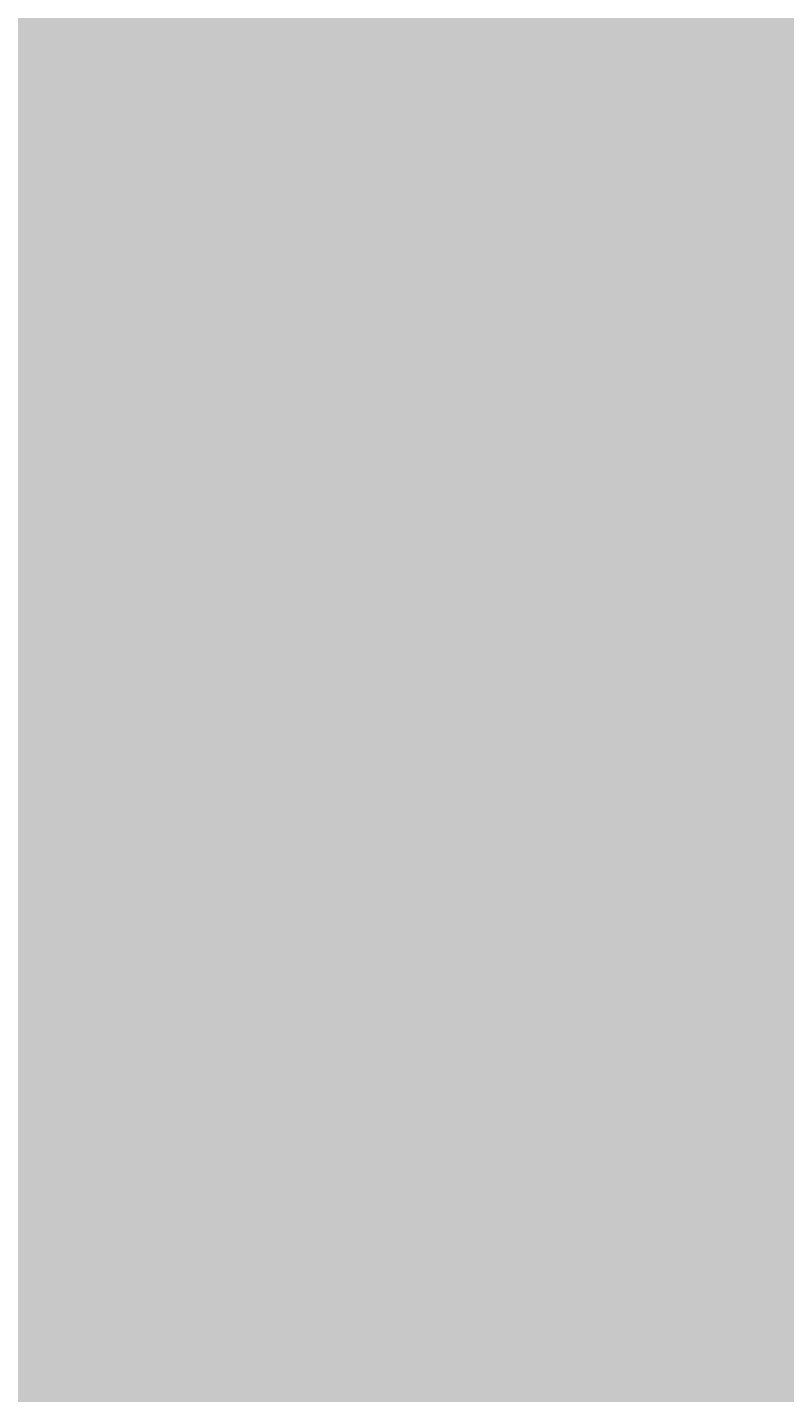
# Model space of a CAD drawing. Units: inches. Extents: x 84 to 1044, y -280 to 906.
# Tile 98 of 105: x 826 to 861, y 445 to 510. Entities that reach past the tile are written whole.
import ezdxf

# ---------------------------------------------------------------- set-up
doc = ezdxf.new("R2010")
doc.units = ezdxf.units.IN
doc.layers.add('A-ANNO-DIMS', color=2, linetype='Continuous', lineweight=18)
doc.layers.add('L-PLNT-PATT', color=9, linetype='Continuous', lineweight=9, true_color=0xafd9aa)
doc.styles.get("Standard").update_dxf_attribs({"font": 'arial.ttf'})
doc.dimstyles.get("Standard").update_dxf_attribs({"dimtxt": 0.18, "dimasz": 0.18, "dimexe": 0.18, "dimexo": 0.0625, "dimgap": 0.09, "dimtad": 0, "dimtih": 1, "dimtoh": 1, "dimdec": 4, "dimzin": 0, "dimdsep": 46, "dimtxsty": 'Standard', "dimcen": 0.09, "dimadec": 0, "dimazin": 0, "dimtfac": 1, "dimtdec": 4, "dimtofl": 0, "dimtmove": 0, "dimatfit": 3, "dimfxl": 1, "dimtolj": 1, "dimtzin": 0, "dimarcsym": 0})

# ---------------------------------------------------------------- blocks, each defined once
blk = doc.blocks.new('*D62')
at = {"layer": 'A-ANNO-DIMS', "color": 0, "lineweight": -2, "transparency": 16777216}
for p, q in [((203.179, 709.183), (203.179, 905.9)), ((203.359, 905.72), (549.232, 905.72)), ((895.894, 905.72), (550.021, 905.72)), ((896.074, 400.183), (896.074, 905.9))]:
    blk.add_line(p, q, dxfattribs=at)
at = {"layer": 'A-ANNO-DIMS', "color": 0, "transparency": 16777216}
for points in [[(203.359, 905.75), (203.359, 905.69), (203.179, 905.72)], [(895.894, 905.75), (895.894, 905.69), (896.074, 905.72)]]:
    blk.add_solid(points, dxfattribs=at)
at = {"layer": 'Defpoints', "color": 0, "transparency": 16777216}
for p in [(896.074, 905.72), (203.179, 709.12), (896.074, 400.12)]:
    blk.add_point(p, dxfattribs=at)
at = {"layer": 'A-ANNO-DIMS', "color": 0, "transparency": 16777216, "insert": (549.627, 905.72), "char_height": 0.18, "attachment_point": 5}
blk.add_mtext('\\A1;692.9', dxfattribs=at)
blk = doc.blocks.new('*D63')
at = {"layer": 'A-ANNO-DIMS', "color": 0, "lineweight": -2, "transparency": 16777216}
for p, q in [((833.136, 709.12), (1043.768, 709.12)), ((1043.588, 708.94), (1043.588, 400.302)), ((1043.588, 91.3), (1043.588, 399.938)), ((896.136, 91.12), (1043.768, 91.12))]:
    blk.add_line(p, q, dxfattribs=at)
at = {"layer": 'A-ANNO-DIMS', "color": 0, "transparency": 16777216}
for points in [[(1043.558, 708.94), (1043.618, 708.94), (1043.588, 709.12)], [(1043.558, 91.3), (1043.618, 91.3), (1043.588, 91.12)]]:
    blk.add_solid(points, dxfattribs=at)
at = {"layer": 'Defpoints', "color": 0, "transparency": 16777216}
for p in [(833.074, 709.12), (1043.588, 709.12), (896.074, 91.12)]:
    blk.add_point(p, dxfattribs=at)
at = {"layer": 'A-ANNO-DIMS', "color": 0, "transparency": 16777216, "insert": (1043.588, 400.12), "char_height": 0.18, "attachment_point": 5}
blk.add_mtext('\\A1;618', dxfattribs=at)

msp = doc.modelspace()

# ---------------------------------------------------------------- hatches: boundary and pattern name
at = {"layer": 'L-PLNT-PATT', "transparency": 33554597}
h = msp.add_hatch(color=256, dxfattribs=at)
h.dxf.hatch_style = 1
h.paths.add_polyline_path([(896.074, 511.12), (704.074, 511.12), (704.074, 491.62), (704.074, 419.62), (704.074, 400.12), (833.074, 400.12), (896.074, 400.12)])

# ---------------------------------------------------------------- dimensions: what is measured, and where the dimension line sits
at = {"layer": 'A-ANNO-DIMS'}
dim = msp.add_linear_dim(base=(896.074, 905.72), p1=(203.179, 709.12), p2=(896.074, 400.12), dimstyle='Standard', override={"dimdec": 1, "dimlfac": 1, "dimrnd": 0, "dimzin": 0, "dimdsep": 46, "dimlunit": 2}, dxfattribs=at)
dim.commit()
dim.dimension.update_dxf_attribs({"geometry": '*D62', "text_midpoint": (549.627, 905.72)})
dim = msp.add_linear_dim(base=(1043.588, 709.12), p1=(896.074, 91.12), p2=(833.074, 709.12), angle=90, dimstyle='Standard', override={"dimdec": 0, "dimlfac": 1, "dimrnd": 0, "dimzin": 0, "dimdsep": 46, "dimlunit": 2}, dxfattribs=at)
dim.commit()
dim.dimension.update_dxf_attribs({"geometry": '*D63', "text_midpoint": (1043.588, 400.12)})

doc.saveas('drawing.dxf')
